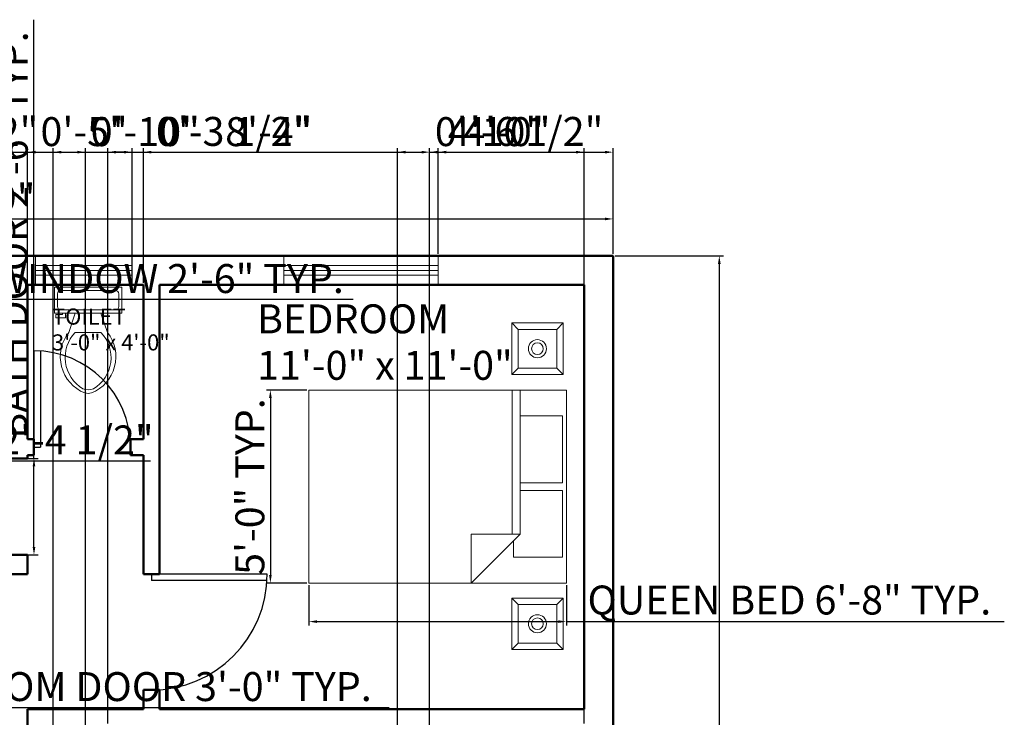
# Model space of a CAD drawing. Units: inches. Extents: x 2866 to 3545, y 873 to 1597.
# Tile 5 of 5: x 3239 to 3545, y 1380 to 1597. Entities that reach past the tile are written whole.
import ezdxf

# ---------------------------------------------------------------- set-up
doc = ezdxf.new("R2010")
doc.units = ezdxf.units.IN
doc.layers.add('A-ANNO-DIMS', color=152, linetype='Continuous', lineweight=18, true_color=0x2776bb)
for name, color, linetype, lineweight in [('A-AREA-IDEN', 7, 'Continuous', 25), ('A-DOOR', 3, 'Continuous', 25), ('A-FLOR-FIXT', 9, 'Continuous', 18), ('A-FURN', 8, 'Continuous', 18), ('A-GLAZ', 4, 'Continuous', 18), ('A-WALL', 7, 'Continuous', 50)]:
    doc.layers.add(name, color=color, linetype=linetype, lineweight=lineweight)
doc.styles.get("Standard").update_dxf_attribs({"font": 'arial.ttf'})
doc.dimstyles.new('ISO-25', dxfattribs={"dimtxt": 9, "dimasz": 2.5, "dimexe": 1.25, "dimexo": 0.625, "dimtad": 1, "dimdec": 0, "dimlunit": 3, "dimtxsty": 'Standard', "dimcen": 4.5, "dimadec": 0, "dimazin": 0, "dimtfac": 1, "dimtdec": 0, "dimtmove": 0, "dimatfit": 3, "dimfxl": 1, "dimarcsym": 0})

# ---------------------------------------------------------------- blocks, each defined once
blk = doc.blocks.new('Bed - Queen')
for p, q in [((0, -80.00003), (0, 0)), ((0, 0), (59.99999, 0)), ((59.99999, 0), (59.99999, -80.00003)), ((7.99999, -1.2), (28.79998, -1.2)), ((7.99999, -14.4), (7.99999, -1.2)), ((28.79998, -1.2), (28.79998, -14.4)), ((31.19999, -1.2), (51.99999, -1.2)), ((31.19999, -14.4), (31.19999, -1.2)), ((51.99999, -1.2), (51.99999, -16.4)), ((0, -14.4), (44.8, -14.4)), ((59.99999, -29.6), (44.8, -14.4)), ((44.8, -14.4), (44.8, -29.6)), ((44.8, -16.8), (0, -16.8)), ((51.99999, -16.4), (46.79936, -16.4)), ((44.8, -29.6), (59.99999, -29.6)), ((59.99999, -80.00003), (0, -80.00003))]:
    blk.add_line(p, q)
blk = doc.blocks.new('Toilet - top')
for p, q in [((9.5, -6), (9.5, -2)), ((-10, -8.5), (-8, -8.5)), ((-10, -9.5), (-10, -8.5)), ((-8, -8.5), (-8, -8)), ((-7, -8), (-7, -9.5)), ((-4, -8), (-6, -14)), ((4, -8), (6, -14)), ((-7, -9.5), (-10, -9.5)), ((4, -14), (-4, -14))]:
    blk.add_line(p, q)
blk.add_lwpolyline([(10.5, -8), (10.5, 0), (-10.5, 0), (-10.5, -8)], close=True)
for points in [[(-9.5, -2), (-9.5, -6)], [(8.5, -1), (-8.5, -1)], [(-8.5, -7), (8.5, -7)]]:
    blk.add_lwpolyline(points)
for centre, radius, start, end in [((-8.62, -1.88), 0.884, 81.8699, 188.1301), ((8.62, -1.88), 0.884, 351.8699, 98.1301), ((-8.62, -6.12), 0.884, 171.8699, 278.1301), ((8.62, -6.12), 0.884, 261.8699, 8.1301), ((3.52, -21.58), 12.17, 141.4691, 247.9714), ((4.2, -21.82), 11.33, 136.3677, 238.9468), ((-3.52, -21.58), 12.17, 292.0284, 38.5307), ((-4.2, -21.82), 11.33, 301.053, 43.6321), ((0, -27.88), 4, 245.7318, 294.2682), ((0, -29), 4, 254.8605, 285.1395)]:
    blk.add_arc(centre, radius, start, end)
blk = doc.blocks.new('*D19')
at = {"layer": 'A-ANNO-DIMS', "color": 0, "lineweight": -2, "transparency": 16777216}
for p, q in [((3423.67, 1523.69), (3457.33, 1523.69)), ((3456.08, 1521.19), (3456.08, 916.19)), ((3423.67, 913.69), (3457.33, 913.69))]:
    blk.add_line(p, q, dxfattribs=at)
at = {"layer": 'A-ANNO-DIMS', "color": 0, "transparency": 16777216}
for points in [[(3455.66, 1521.19), (3456.5, 1521.19), (3456.08, 1523.69)], [(3455.66, 916.19), (3456.5, 916.19), (3456.08, 913.69)]]:
    blk.add_solid(points, dxfattribs=at)
at = {"layer": 'Defpoints', "color": 0, "transparency": 16777216}
for p in [(3423.04, 1523.69), (3423.04, 913.69), (3456.08, 913.69)]:
    blk.add_point(p, dxfattribs=at)
at = {"layer": 'A-ANNO-DIMS', "color": 0, "transparency": 16777216, "insert": (3450.86, 1218.69), "char_height": 9, "attachment_point": 5, "rotation": 90}
blk.add_mtext('50\'-10"', dxfattribs=at)
blk = doc.blocks.new('*D20')
at = {"layer": 'A-ANNO-DIMS', "color": 0, "lineweight": -2, "transparency": 16777216}
for p, q in [((3030.04, 1524.32), (3030.04, 1536.42)), ((3032.54, 1535.17), (3420.54, 1535.17)), ((3423.04, 1524.32), (3423.04, 1536.42))]:
    blk.add_line(p, q, dxfattribs=at)
at = {"layer": 'A-ANNO-DIMS', "color": 0, "transparency": 16777216}
for points in [[(3032.54, 1535.59), (3032.54, 1534.76), (3030.04, 1535.17)], [(3420.54, 1535.59), (3420.54, 1534.76), (3423.04, 1535.17)]]:
    blk.add_solid(points, dxfattribs=at)
at = {"layer": 'Defpoints', "color": 0, "transparency": 16777216}
for p in [(3423.04, 1535.17), (3030.04, 1523.69), (3423.04, 1523.69)]:
    blk.add_point(p, dxfattribs=at)
at = {"layer": 'A-ANNO-DIMS', "color": 0, "transparency": 16777216, "insert": (3226.54, 1540.4), "char_height": 9, "attachment_point": 5}
blk.add_mtext('32\'-9"', dxfattribs=at)
blk = doc.blocks.new('WIN-48IN')
for p, q in [((0, 0), (0, 48)), ((0, 48), (9, 48)), ((3, 0), (3, 48)), ((4.5, 0), (4.5, 48)), ((6, 0), (6, 48)), ((9, 48), (9, 0)), ((9, 0), (0, 0))]:
    blk.add_line(p, q)
blk = doc.blocks.new('WIN-30IN')
for p, q in [((0, 0), (0, 30)), ((0, 30), (9, 30)), ((3, 0), (3, 30)), ((4.5, 0), (4.5, 30)), ((6, 0), (6, 30)), ((9, 30), (9, 0)), ((9, 0), (0, 0))]:
    blk.add_line(p, q)
blk = doc.blocks.new('BEDSIDE-STAND-16IN')
for p, q in [((0, 16), (2, 14)), ((14, 14), (16, 16)), ((0, 0), (2, 2)), ((16, 0), (14, 2))]:
    blk.add_line(p, q)
for points in [[(0, 16), (16, 16), (16, 0), (0, 0)], [(2, 14), (14, 14), (14, 2), (2, 2)]]:
    blk.add_lwpolyline(points, close=True)
for radius in [2.82, 1.82]:
    blk.add_circle((8, 8), radius)
blk = doc.blocks.new('DOOR-SWING-30IN')
for p, q in [((0, 30), (0, 0)), ((2, 30), (2, 0)), ((0, 0), (2, 0))]:
    blk.add_line(p, q)
blk.add_arc((0, 0), 30, 0, 90)
blk = doc.blocks.new('DOOR-SWING-36IN')
for p, q in [((0, 2), (36, 2)), ((36, 0), (36, 2)), ((0, 0), (36, 0))]:
    blk.add_line(p, q)
blk.add_arc((36, 0), 36, 90, 180)
blk = doc.blocks.new('*D29')
at = {"layer": 'A-ANNO-DIMS', "color": 0, "lineweight": -2, "transparency": 16777216}
for p, q in [((3194.66, 1514.07), (3194.66, 1508.94)), ((3224.66, 1514.07), (3224.66, 1508.94)), ((3197.16, 1510.19), (3222.16, 1510.19)), ((3224.66, 1510.19), (3342.29, 1510.19))]:
    blk.add_line(p, q, dxfattribs=at)
at = {"layer": 'A-ANNO-DIMS', "color": 0, "transparency": 16777216}
for points in [[(3197.16, 1510.61), (3197.16, 1509.78), (3194.66, 1510.19)], [(3222.16, 1510.61), (3222.16, 1509.78), (3224.66, 1510.19)]]:
    blk.add_solid(points, dxfattribs=at)
at = {"layer": 'Defpoints', "color": 0, "transparency": 16777216}
for p in [(3194.66, 1514.69), (3224.66, 1514.69), (3224.66, 1510.19)]:
    blk.add_point(p, dxfattribs=at)
at = {"layer": 'A-ANNO-DIMS', "color": 0, "transparency": 16777216, "insert": (3284.73, 1515.47), "char_height": 9, "attachment_point": 5}
blk.add_mtext('WINDOW 2\'-6" TYP.', dxfattribs=at)
blk = doc.blocks.new('*D33')
at = {"layer": 'A-ANNO-DIMS', "color": 0, "lineweight": -2, "transparency": 16777216}
for p, q in [((3328.53, 1421.32), (3328.53, 1408.7)), ((3408.53, 1421.32), (3408.53, 1408.7)), ((3331.03, 1409.95), (3406.03, 1409.95)), ((3408.53, 1409.95), (3544.67, 1409.95))]:
    blk.add_line(p, q, dxfattribs=at)
at = {"layer": 'A-ANNO-DIMS', "color": 0, "transparency": 16777216}
for points in [[(3331.03, 1410.37), (3331.03, 1409.53), (3328.53, 1409.95)], [(3406.03, 1410.37), (3406.03, 1409.53), (3408.53, 1409.95)]]:
    blk.add_solid(points, dxfattribs=at)
at = {"layer": 'Defpoints', "color": 0, "transparency": 16777216}
for p in [(3328.53, 1421.95), (3408.53, 1421.95), (3408.53, 1409.95)]:
    blk.add_point(p, dxfattribs=at)
at = {"layer": 'A-ANNO-DIMS', "color": 0, "transparency": 16777216, "insert": (3477.85, 1415.5), "char_height": 9, "attachment_point": 5}
blk.add_mtext('QUEEN BED 6\'-8" TYP.', dxfattribs=at)
blk = doc.blocks.new('*D34')
at = {"layer": 'A-ANNO-DIMS', "color": 0, "lineweight": -2, "transparency": 16777216}
for p, q in [((3327.9, 1481.95), (3315.28, 1481.95)), ((3316.53, 1479.45), (3316.53, 1424.45)), ((3327.9, 1421.95), (3315.28, 1421.95))]:
    blk.add_line(p, q, dxfattribs=at)
at = {"layer": 'A-ANNO-DIMS', "color": 0, "transparency": 16777216}
for points in [[(3316.11, 1479.45), (3316.95, 1479.45), (3316.53, 1481.95)], [(3316.11, 1424.45), (3316.95, 1424.45), (3316.53, 1421.95)]]:
    blk.add_solid(points, dxfattribs=at)
at = {"layer": 'Defpoints', "color": 0, "transparency": 16777216}
for p in [(3328.53, 1481.95), (3316.53, 1421.95), (3328.53, 1421.95)]:
    blk.add_point(p, dxfattribs=at)
at = {"layer": 'A-ANNO-DIMS', "color": 0, "transparency": 16777216, "insert": (3311.31, 1451.95), "char_height": 9, "attachment_point": 5, "rotation": 90}
blk.add_mtext('5\'-0" TYP.', dxfattribs=at)
blk = doc.blocks.new('*D35')
at = {"layer": 'A-ANNO-DIMS', "color": 0, "lineweight": -2, "transparency": 16777216}
for p, q in [((3243.04, 1460.69), (3243.04, 1597.14)), ((3239.17, 1460.69), (3244.29, 1460.69)), ((3243.04, 1433.19), (3243.04, 1458.19)), ((3239.17, 1430.69), (3244.29, 1430.69))]:
    blk.add_line(p, q, dxfattribs=at)
at = {"layer": 'A-ANNO-DIMS', "color": 0, "transparency": 16777216}
for points in [[(3242.63, 1458.19), (3243.46, 1458.19), (3243.04, 1460.69)], [(3242.63, 1433.19), (3243.46, 1433.19), (3243.04, 1430.69)]]:
    blk.add_solid(points, dxfattribs=at)
at = {"layer": 'Defpoints', "color": 0, "transparency": 16777216}
for p in [(3238.54, 1460.69), (3243.04, 1460.69), (3238.54, 1430.69)]:
    blk.add_point(p, dxfattribs=at)
at = {"layer": 'A-ANNO-DIMS', "color": 0, "transparency": 16777216, "insert": (3237.76, 1530.17), "char_height": 9, "attachment_point": 5, "rotation": 90}
blk.add_mtext('BATH DOOR 2\'-6" TYP.', dxfattribs=at)
blk = doc.blocks.new('*D37')
at = {"layer": 'A-ANNO-DIMS', "color": 0, "lineweight": -2, "transparency": 16777216}
for p, q in [((3149.54, 1388.07), (3149.54, 1382.04)), ((3185.54, 1388.07), (3185.54, 1382.04)), ((3152.04, 1383.29), (3183.04, 1383.29)), ((3185.54, 1383.29), (3353.42, 1383.29))]:
    blk.add_line(p, q, dxfattribs=at)
at = {"layer": 'A-ANNO-DIMS', "color": 0, "transparency": 16777216}
for points in [[(3152.04, 1383.71), (3152.04, 1382.88), (3149.54, 1383.29)], [(3183.04, 1383.71), (3183.04, 1382.88), (3185.54, 1383.29)]]:
    blk.add_solid(points, dxfattribs=at)
at = {"layer": 'Defpoints', "color": 0, "transparency": 16777216}
for p in [(3149.54, 1388.69), (3185.54, 1388.69), (3185.54, 1383.29)]:
    blk.add_point(p, dxfattribs=at)
at = {"layer": 'A-ANNO-DIMS', "color": 0, "transparency": 16777216, "insert": (3270.73, 1388.58), "char_height": 9, "attachment_point": 5}
blk.add_mtext('BEDROOM DOOR 3\'-0" TYP.', dxfattribs=at)
blk = doc.blocks.new('*D58')
at = {"layer": 'A-ANNO-DIMS', "color": 0, "lineweight": -2, "transparency": 16777216}
for p, q in [((3201.88, 1466.51), (3201.88, 1458.75)), ((3230.42, 1466.51), (3230.42, 1458.75)), ((3204.38, 1460), (3227.92, 1460)), ((3230.42, 1460), (3279.22, 1460))]:
    blk.add_line(p, q, dxfattribs=at)
at = {"layer": 'A-ANNO-DIMS', "color": 0, "transparency": 16777216}
for points in [[(3204.38, 1460.42), (3204.38, 1459.59), (3201.88, 1460)], [(3227.92, 1460.42), (3227.92, 1459.59), (3230.42, 1460)]]:
    blk.add_solid(points, dxfattribs=at)
at = {"layer": 'Defpoints', "color": 0, "transparency": 16777216}
for p in [(3201.88, 1467.14), (3230.42, 1467.14), (3230.42, 1460)]:
    blk.add_point(p, dxfattribs=at)
at = {"layer": 'A-ANNO-DIMS', "color": 0, "transparency": 16777216, "insert": (3256.07, 1465.28), "char_height": 9, "attachment_point": 5}
blk.add_mtext('2\'-4 1/2"', dxfattribs=at)
blk = doc.blocks.new('*D64')
at = {"layer": 'A-ANNO-DIMS', "color": 0, "lineweight": -2, "transparency": 16777216}
for p, q in [((3368.69, 1524.32), (3368.69, 1557.19)), ((3371.19, 1555.94), (3420.54, 1555.94)), ((3423.04, 1524.32), (3423.04, 1557.19))]:
    blk.add_line(p, q, dxfattribs=at)
at = {"layer": 'A-ANNO-DIMS', "color": 0, "transparency": 16777216}
for points in [[(3371.19, 1556.36), (3371.19, 1555.53), (3368.69, 1555.94)], [(3420.54, 1556.36), (3420.54, 1555.53), (3423.04, 1555.94)]]:
    blk.add_solid(points, dxfattribs=at)
at = {"layer": 'Defpoints', "color": 0, "transparency": 16777216}
for p in [(3423.04, 1555.94), (3368.69, 1523.69), (3423.04, 1523.69)]:
    blk.add_point(p, dxfattribs=at)
at = {"layer": 'A-ANNO-DIMS', "color": 0, "transparency": 16777216, "insert": (3395.87, 1561.22), "char_height": 9, "attachment_point": 5}
blk.add_mtext('4\'-6 1/2"', dxfattribs=at)
blk = doc.blocks.new('*D65')
at = {"layer": 'A-ANNO-DIMS', "color": 0, "lineweight": -2, "transparency": 16777216}
for p, q in [((3188.04, 1515.32), (3188.04, 1557.19)), ((3190.54, 1555.94), (3192.16, 1555.94)), ((3194.66, 1515.32), (3194.66, 1557.19)), ((3194.66, 1555.94), (3243.3, 1555.94))]:
    blk.add_line(p, q, dxfattribs=at)
at = {"layer": 'A-ANNO-DIMS', "color": 0, "transparency": 16777216}
for points in [[(3190.54, 1556.36), (3190.54, 1555.53), (3188.04, 1555.94)], [(3192.16, 1556.36), (3192.16, 1555.53), (3194.66, 1555.94)]]:
    blk.add_solid(points, dxfattribs=at)
at = {"layer": 'Defpoints', "color": 0, "transparency": 16777216}
for p in [(3194.66, 1555.94), (3188.04, 1514.69), (3194.66, 1514.69)]:
    blk.add_point(p, dxfattribs=at)
at = {"layer": 'A-ANNO-DIMS', "color": 0, "transparency": 16777216, "insert": (3220.23, 1561.22), "char_height": 9, "attachment_point": 5}
blk.add_mtext('0\'-6 1/2"', dxfattribs=at)
blk = doc.blocks.new('*D66')
at = {"layer": 'A-ANNO-DIMS', "color": 0, "lineweight": -2, "transparency": 16777216}
for p, q in [((3271.02, 1555.94), (3268.52, 1555.94)), ((3273.52, 1515.32), (3273.52, 1557.19)), ((3273.52, 1555.94), (3277.04, 1555.94)), ((3277.04, 1515.32), (3277.04, 1557.19)), ((3279.54, 1555.94), (3328.19, 1555.94))]:
    blk.add_line(p, q, dxfattribs=at)
at = {"layer": 'A-ANNO-DIMS', "color": 0, "transparency": 16777216}
for points in [[(3271.02, 1556.36), (3271.02, 1555.53), (3273.52, 1555.94)], [(3279.54, 1556.36), (3279.54, 1555.53), (3277.04, 1555.94)]]:
    blk.add_solid(points, dxfattribs=at)
at = {"layer": 'Defpoints', "color": 0, "transparency": 16777216}
for p in [(3277.04, 1555.94), (3273.52, 1514.69), (3277.04, 1514.69)]:
    blk.add_point(p, dxfattribs=at)
at = {"layer": 'A-ANNO-DIMS', "color": 0, "transparency": 16777216, "insert": (3305.11, 1561.22), "char_height": 9, "attachment_point": 5}
blk.add_mtext('0\'-3 1/2"', dxfattribs=at)
blk = doc.blocks.new('*D67')
at = {"layer": 'A-ANNO-DIMS', "color": 0, "lineweight": -2, "transparency": 16777216}
for p, q in [((3233.54, 1555.94), (3231.04, 1555.94)), ((3236.04, 1515.32), (3236.04, 1557.19)), ((3236.04, 1555.94), (3241.04, 1555.94)), ((3241.04, 1515.32), (3241.04, 1557.19)), ((3243.54, 1555.94), (3271.22, 1555.94))]:
    blk.add_line(p, q, dxfattribs=at)
at = {"layer": 'A-ANNO-DIMS', "color": 0, "transparency": 16777216}
for points in [[(3233.54, 1556.36), (3233.54, 1555.53), (3236.04, 1555.94)], [(3243.54, 1556.36), (3243.54, 1555.53), (3241.04, 1555.94)]]:
    blk.add_solid(points, dxfattribs=at)
at = {"layer": 'Defpoints', "color": 0, "transparency": 16777216}
for p in [(3241.04, 1555.94), (3236.04, 1514.69), (3241.04, 1514.69)]:
    blk.add_point(p, dxfattribs=at)
at = {"layer": 'A-ANNO-DIMS', "color": 0, "transparency": 16777216, "insert": (3258.63, 1561.16), "char_height": 9, "attachment_point": 5}
blk.add_mtext('0\'-5"', dxfattribs=at)
blk = doc.blocks.new('*D80')
at = {"layer": 'A-ANNO-DIMS', "color": 0, "lineweight": -2, "transparency": 16777216}
for p, q in [((3249.04, 1088.32), (3249.04, 1557.19)), ((3251.54, 1555.94), (3256.54, 1555.94)), ((3259.04, 1088.32), (3259.04, 1557.19)), ((3259.04, 1555.94), (3293.71, 1555.94))]:
    blk.add_line(p, q, dxfattribs=at)
at = {"layer": 'A-ANNO-DIMS', "color": 0, "transparency": 16777216}
for points in [[(3251.54, 1556.36), (3251.54, 1555.53), (3249.04, 1555.94)], [(3256.54, 1556.36), (3256.54, 1555.53), (3259.04, 1555.94)]]:
    blk.add_solid(points, dxfattribs=at)
at = {"layer": 'Defpoints', "color": 0, "transparency": 16777216}
for p in [(3259.04, 1555.94), (3249.04, 1087.69), (3259.04, 1087.69)]:
    blk.add_point(p, dxfattribs=at)
at = {"layer": 'A-ANNO-DIMS', "color": 0, "transparency": 16777216, "insert": (3277.63, 1561.16), "char_height": 9, "attachment_point": 5}
blk.add_mtext('0\'-10"', dxfattribs=at)
blk = doc.blocks.new('*D81')
at = {"layer": 'A-ANNO-DIMS', "color": 0, "lineweight": -2, "transparency": 16777216}
for p, q in [((3266.04, 1378.32), (3266.04, 1557.19)), ((3268.54, 1555.94), (3363.54, 1555.94)), ((3366.04, 1378.32), (3366.04, 1557.19))]:
    blk.add_line(p, q, dxfattribs=at)
at = {"layer": 'A-ANNO-DIMS', "color": 0, "transparency": 16777216}
for points in [[(3268.54, 1556.36), (3268.54, 1555.53), (3266.04, 1555.94)], [(3363.54, 1556.36), (3363.54, 1555.53), (3366.04, 1555.94)]]:
    blk.add_solid(points, dxfattribs=at)
at = {"layer": 'Defpoints', "color": 0, "transparency": 16777216}
for p in [(3366.04, 1555.94), (3266.04, 1377.69), (3366.04, 1377.69)]:
    blk.add_point(p, dxfattribs=at)
at = {"layer": 'A-ANNO-DIMS', "color": 0, "transparency": 16777216, "insert": (3316.04, 1561.16), "char_height": 9, "attachment_point": 5}
blk.add_mtext('8\'-4"', dxfattribs=at)
blk = doc.blocks.new('*D82')
at = {"layer": 'A-ANNO-DIMS', "color": 0, "lineweight": -2, "transparency": 16777216}
for p, q in [((3366.04, 1378.32), (3366.04, 1557.19)), ((3368.54, 1555.94), (3411.54, 1555.94)), ((3414.04, 1378.32), (3414.04, 1557.19))]:
    blk.add_line(p, q, dxfattribs=at)
at = {"layer": 'A-ANNO-DIMS', "color": 0, "transparency": 16777216}
for points in [[(3368.54, 1556.36), (3368.54, 1555.53), (3366.04, 1555.94)], [(3411.54, 1556.36), (3411.54, 1555.53), (3414.04, 1555.94)]]:
    blk.add_solid(points, dxfattribs=at)
at = {"layer": 'Defpoints', "color": 0, "transparency": 16777216}
for p in [(3414.04, 1555.94), (3366.04, 1377.69), (3414.04, 1377.69)]:
    blk.add_point(p, dxfattribs=at)
at = {"layer": 'A-ANNO-DIMS', "color": 0, "transparency": 16777216, "insert": (3390.04, 1561.16), "char_height": 9, "attachment_point": 5}
blk.add_mtext('4\'-0"', dxfattribs=at)
blk = doc.blocks.new('*D83')
at = {"layer": 'A-ANNO-DIMS', "color": 0, "lineweight": -2, "transparency": 16777216}
for p, q in [((3356.04, 1330.32), (3356.04, 1557.19)), ((3358.54, 1555.94), (3363.54, 1555.94)), ((3366.04, 1330.32), (3366.04, 1557.19)), ((3366.04, 1555.94), (3400.71, 1555.94))]:
    blk.add_line(p, q, dxfattribs=at)
at = {"layer": 'A-ANNO-DIMS', "color": 0, "transparency": 16777216}
for points in [[(3358.54, 1556.36), (3358.54, 1555.53), (3356.04, 1555.94)], [(3363.54, 1556.36), (3363.54, 1555.53), (3366.04, 1555.94)]]:
    blk.add_solid(points, dxfattribs=at)
at = {"layer": 'Defpoints', "color": 0, "transparency": 16777216}
for p in [(3366.04, 1555.94), (3356.04, 1329.69), (3366.04, 1329.69)]:
    blk.add_point(p, dxfattribs=at)
at = {"layer": 'A-ANNO-DIMS', "color": 0, "transparency": 16777216, "insert": (3384.63, 1561.16), "char_height": 9, "attachment_point": 5}
blk.add_mtext('0\'-10"', dxfattribs=at)

msp = doc.modelspace()

# ---------------------------------------------------------------- linework, layer by layer
at = {"layer": 'A-WALL'}
for p, q in [((3030.04, 1523.69), (3423.04, 1523.69)), ((3423.04, 1523.69), (3423.04, 913.69)), ((3241.04, 1514.69), (3241.04, 1466.69)), ((3241.04, 1514.69), (3277.04, 1514.69)), ((3277.04, 1514.69), (3277.04, 1466.69)), ((3282.04, 1514.69), (3282.04, 1424.69)), ((3282.04, 1514.69), (3414.04, 1514.69)), ((3414.04, 1514.69), (3414.04, 1382.69)), ((3241.04, 1466.69), (3243.04, 1466.69)), ((3243.04, 1466.69), (3243.04, 1461.69)), ((3273.04, 1466.69), (3273.04, 1461.69)), ((3273.04, 1466.69), (3277.04, 1466.69)), ((3236.04, 1460.69), (3241.04, 1460.69)), ((3241.04, 1461.69), (3243.04, 1461.69)), ((3241.04, 1461.69), (3241.04, 1460.69)), ((3273.04, 1461.69), (3277.04, 1461.69)), ((3277.04, 1461.69), (3277.04, 1424.69)), ((3188.04, 1430.69), (3241.04, 1430.69)), ((3241.04, 1430.69), (3241.04, 1424.69)), ((3241.04, 1427.69), (3241.04, 1424.69)), ((3183.04, 1424.69), (3241.04, 1424.69)), ((3236.04, 1424.69), (3241.04, 1424.69)), ((3277.04, 1424.69), (3282.04, 1424.69)), ((3277.04, 1424.69), (3282.04, 1424.69)), ((3277.04, 1388.69), (3282.04, 1388.69)), ((3277.04, 1388.69), (3277.04, 1382.69)), ((3282.04, 1388.69), (3282.04, 1382.69)), ((3241.04, 1382.69), (3277.04, 1382.69)), ((3241.04, 1382.69), (3241.04, 1377.69)), ((3282.04, 1382.69), (3414.04, 1382.69))]:
    msp.add_line(p, q, dxfattribs=at)

# ---------------------------------------------------------------- block references
at = {"layer": 'A-DOOR'}
msp.add_blockref('DOOR-SWING-30IN', (3243.04, 1464.19), dxfattribs=at)
at = {"layer": 'A-DOOR', "rotation": 180}
msp.add_blockref('DOOR-SWING-36IN', (3315.54, 1424.69), dxfattribs=at)
at = {"layer": 'A-FLOR-FIXT'}
msp.add_blockref('Toilet - top', (3259.87, 1513.91), dxfattribs=at)
at = {"layer": 'A-FURN'}
for p in [(3391.54, 1486.82), (3391.54, 1401.29)]:
    msp.add_blockref('BEDSIDE-STAND-16IN', p, dxfattribs=at)
at = {"layer": 'A-FURN', "rotation": 270}
msp.add_blockref('Bed - Queen', (3408.53, 1481.95), dxfattribs=at)
at = {"layer": 'A-GLAZ'}
for name, p, rotation in [('WIN-30IN', (3243.53, 1523.69), 270.0000000000005), ('WIN-48IN', (3320.69, 1523.69), 270.0000000000002)]:
    msp.add_blockref(name, p, dxfattribs=dict(at, rotation=rotation))

# ---------------------------------------------------------------- texts
at = {"layer": 'A-AREA-IDEN'}
for s, height, p in [('TOILET', 5, (3248.63, 1502.31)), ('BEDROOM', 9, (3312.38, 1499.61)), ('3\'-0" x 4\'-0"', 5, (3248.63, 1494.28)), ('11\'-0" x 11\'-0"', 9, (3312.38, 1485.15))]:
    msp.add_text(s, height=height, dxfattribs=at).set_placement(p)

# ---------------------------------------------------------------- dimensions: what is measured, and where the dimension line sits
at = {"layer": 'A-ANNO-DIMS'}
for base, p1, p2, angle, text, picture, middle in [((3243.04, 1460.69), (3238.54, 1430.69), (3238.54, 1460.69), 90, 'BATH DOOR <> TYP.', '*D35', (3237.76, 1530.17)), ((3316.53, 1421.95), (3328.53, 1481.95), (3328.53, 1421.95), 270, '<> TYP.', '*D34', (3311.31, 1451.95))]:
    dim = msp.add_linear_dim(base=base, p1=p1, p2=p2, angle=angle, text=text, dimstyle='ISO-25', override={"dimdec": 1, "dimlfac": 1, "dimrnd": 0, "dimzin": 1, "dimdsep": 46, "dimlunit": 4, "dimfrac": 2}, dxfattribs=at)
    dim.commit()
    dim.dimension.update_dxf_attribs({"geometry": picture, "text_midpoint": middle})
for base, p1, p2, override, picture, middle in [((3194.66, 1555.94), (3188.04, 1514.69), (3194.66, 1514.69), {"dimdec": 1, "dimlfac": 1, "dimrnd": 0, "dimzin": 1, "dimdsep": 46, "dimlunit": 4, "dimfrac": 2}, '*D65', (3220.23, 1561.22)), ((3277.04, 1555.94), (3273.52, 1514.69), (3277.04, 1514.69), {"dimdec": 1, "dimlfac": 1, "dimrnd": 0, "dimzin": 1, "dimdsep": 46, "dimlunit": 4, "dimfrac": 2}, '*D66', (3305.11, 1561.22)), ((3423.0417, 1555.9417), (3368.6903, 1523.6917), (3423.0417, 1523.6917), {"dimdec": 1, "dimlfac": 1, "dimrnd": 0, "dimzin": 1, "dimdsep": 46, "dimlunit": 4, "dimfrac": 2}, '*D64', (3395.866, 1561.2202)), ((3241.04, 1555.94), (3236.04, 1514.69), (3241.04, 1514.69), {"dimdec": 1, "dimlfac": 1, "dimrnd": 0, "dimzin": 1, "dimdsep": 46, "dimlunit": 4, "dimfrac": 2}, '*D67', (3258.63, 1561.16)), ((3259.04, 1555.94), (3249.04, 1087.69), (3259.04, 1087.69), {"dimdec": 1, "dimlfac": 1, "dimrnd": 0, "dimzin": 1, "dimdsep": 46, "dimlunit": 4, "dimfrac": 2}, '*D80', (3277.63, 1561.16)), ((3366.04, 1555.94), (3266.04, 1377.69), (3366.04, 1377.69), {"dimdec": 1, "dimlfac": 1, "dimrnd": 0, "dimzin": 1, "dimdsep": 46, "dimlunit": 4, "dimfrac": 2}, '*D81', (3316.04, 1561.16)), ((3366.04, 1555.94), (3356.04, 1329.69), (3366.04, 1329.69), {"dimdec": 1, "dimlfac": 1, "dimrnd": 0, "dimzin": 1, "dimdsep": 46, "dimlunit": 4, "dimfrac": 2}, '*D83', (3384.63, 1561.16)), ((3414.04, 1555.94), (3366.04, 1377.69), (3414.04, 1377.69), {"dimdec": 1, "dimlfac": 1, "dimrnd": 0, "dimzin": 1, "dimdsep": 46, "dimlunit": 4, "dimfrac": 2}, '*D82', (3390.04, 1561.16)), ((3423.04, 1535.17), (3030.04, 1523.69), (3423.04, 1523.69), {"dimclrd": 0, "dimclre": 0, "dimclrt": 0}, '*D20', (3226.54, 1540.4)), ((3230.42, 1460), (3201.88, 1467.14), (3230.42, 1467.14), {"dimdec": 1, "dimlfac": 1, "dimrnd": 0, "dimzin": 1, "dimdsep": 46, "dimlunit": 4, "dimfrac": 2}, '*D58', (3256.07, 1465.28))]:
    dim = msp.add_linear_dim(base=base, p1=p1, p2=p2, dimstyle='ISO-25', override=override, dxfattribs=at)
    dim.commit()
    dim.dimension.update_dxf_attribs({"geometry": picture, "text_midpoint": middle})
for base, p1, p2, text, picture, middle in [((3224.66, 1510.19), (3194.66, 1514.69), (3224.66, 1514.69), 'WINDOW <> TYP.', '*D29', (3284.73, 1515.47)), ((3408.53, 1409.95), (3328.53, 1421.95), (3408.53, 1421.95), 'QUEEN BED <> TYP.', '*D33', (3477.85, 1415.5)), ((3185.54, 1383.29), (3149.54, 1388.69), (3185.54, 1388.69), 'BEDROOM DOOR <> TYP.', '*D37', (3270.73, 1388.58))]:
    dim = msp.add_linear_dim(base=base, p1=p1, p2=p2, text=text, dimstyle='ISO-25', override={"dimdec": 1, "dimlfac": 1, "dimrnd": 0, "dimzin": 1, "dimdsep": 46, "dimlunit": 4, "dimfrac": 2}, dxfattribs=at)
    dim.commit()
    dim.dimension.update_dxf_attribs({"geometry": picture, "text_midpoint": middle})
dim = msp.add_linear_dim(base=(3456.08, 913.69), p1=(3423.04, 1523.69), p2=(3423.04, 913.69), angle=90, dimstyle='ISO-25', override={"dimclrd": 0, "dimclre": 0, "dimclrt": 0}, dxfattribs=at)
dim.commit()
dim.dimension.update_dxf_attribs({"geometry": '*D19', "text_midpoint": (3450.86, 1218.69)})

doc.saveas('drawing.dxf')
